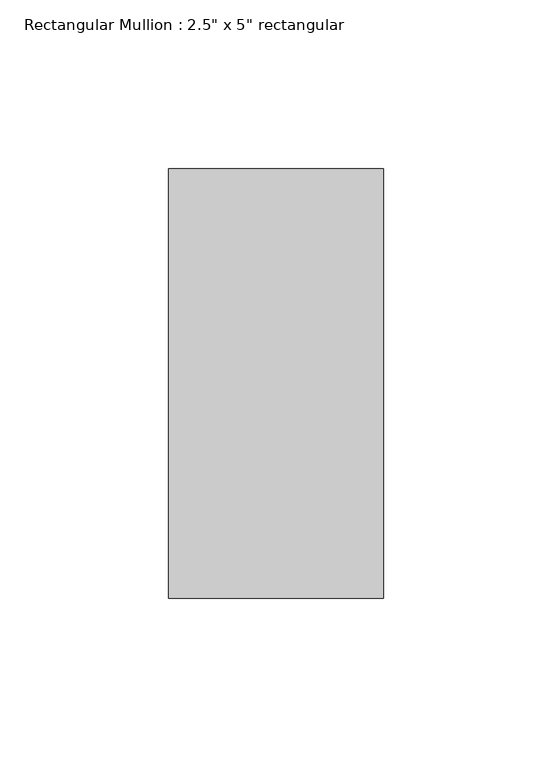
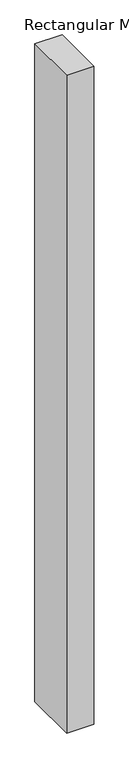
"""IFC4 building model written with IfcOpenShell, lengths in millimetres: member geometry."""

from ifc_helpers import new_model, si_unit, frame, origin, place, context, project, spatial, polyline, outline, extrude, source, transform, mapped, element, save


def member_f7075cef(model_context):
    return source(origin(), model_context, "Body", "SweptSolid", [
        extrude(outline(polyline([(0.0, 63.5), (0.0, -63.5), (-63.5, -63.5), (-63.5, 63.5), (0.0, 63.5)])), frame((0.0, 0.0, -1612.9), z_axis=(0.0, 0.0, 1.0), x_axis=(1.0, 0.0, 0.0)), (0.0, 0.0, 1.0), 1612.9),
    ])


if __name__ == "__main__":
    model = new_model("IFC4")
    model_context = context("Model", 3, world=origin())
    ifc_project = project(units=[si_unit("LENGTHUNIT", "METRE", prefix="MILLI")], contexts=[model_context])
    site = spatial("IfcSite", under=ifc_project)
    building = spatial("IfcBuilding", under=site)
    placement = place(None, origin())
    member_shape = member_f7075cef(model_context)
    element("IfcMember", 1, ObjectType="Rectangular Mullion : 2.5\" x 5\" rectangular", at=placement, inside=building, context=model_context, shape_type="MappedRepresentation", body=[
        mapped(member_shape, transform((0.0, 0.0, 0.0), x_axis=(1.0, 0.0, 0.0), y_axis=(0.0, 1.0, 0.0), z_axis=(0.0, 0.0, 1.0))),
    ])
    save(model, "model.ifc")

# Revit data of these elements
# Type "Rectangular Mullion : 2.5\" x 5\" rectangular"
#   built-in parameter 1007304 = 0.416667 (stored number, unit not read)
#   built-in parameter 1007301 = 0.104167 (stored number, unit not read)
#   built-in parameter 1007300 = 0.104167 (stored number, unit not read)
# Element 1 (IfcMember, "Rectangular Mullion : 2.5\" x 5\" rectangular")
#   Materials on its faces: "Aluminum"
# Materials
#   "Aluminum": class "Metal", colour RGB 247 247 247, transparency 0, Description = "Aluminum 6061", Cost = 0
